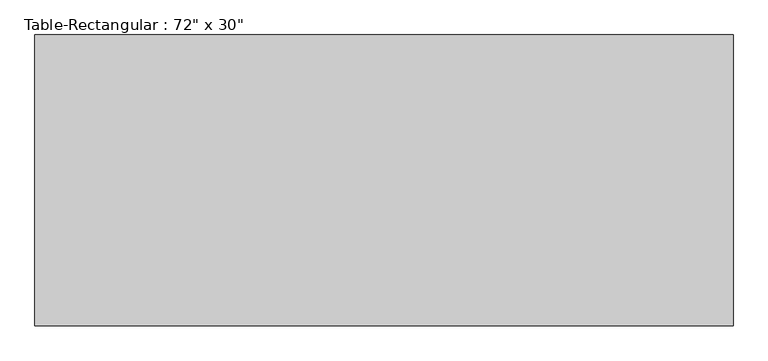
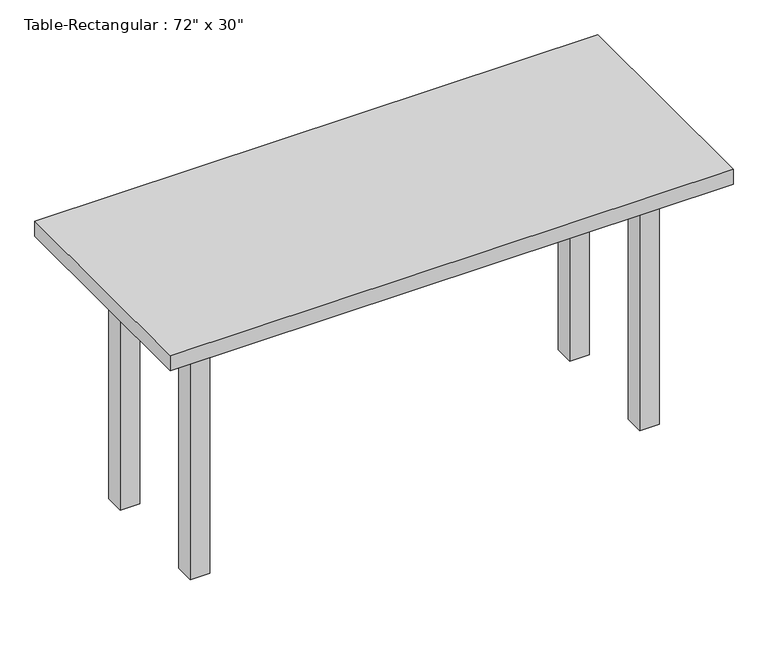
"""IFC4 building model written with IfcOpenShell, lengths in millimetres: furniture geometry."""

from ifc_helpers import new_model, si_unit, frame, origin, origin_with_axes, place, context, project, spatial, polyline, outline, extrude, source, transform, mapped, element, save


def furniture_046c8a23(model_context):
    return source(origin(), model_context, "Body", "SweptSolid", [
        extrude(outline(polyline([(698.5, 190.5), (698.5, 165.1), (-698.5, 165.1), (-698.5, 190.5), (698.5, 190.5)])), frame((0.0, 0.0, 762.0), z_axis=(0.0, 0.0, 1.0), x_axis=(1.0, 0.0, 0.0)), (0.0, 0.0, 1.0), 101.6),
        extrude(outline(polyline([(698.5, -190.5), (-698.5, -190.5), (-698.5, -165.1), (698.5, -165.1), (698.5, -190.5)])), frame((0.0, 0.0, 762.0), z_axis=(0.0, 0.0, 1.0), x_axis=(1.0, 0.0, 0.0)), (0.0, 0.0, 1.0), 101.6),
        extrude(outline(polyline([(-711.2, -165.1), (-736.6, -165.1), (-736.6, 165.1), (-711.2, 165.1), (-711.2, -165.1)])), frame((0.0, 0.0, 762.0), z_axis=(0.0, 0.0, 1.0), x_axis=(1.0, 0.0, 0.0)), (0.0, 0.0, 1.0), 101.6),
        extrude(outline(polyline([(711.2, -165.1), (711.2, 165.1), (736.6, 165.1), (736.6, -165.1), (711.2, -165.1)])), frame((0.0, 0.0, 762.0), z_axis=(0.0, 0.0, 1.0), x_axis=(1.0, 0.0, 0.0)), (0.0, 0.0, 1.0), 101.6),
        extrude(outline(polyline([(914.4, 381.0), (914.4, -381.0), (-914.4, -381.0), (-914.4, 381.0), (914.4, 381.0)])), frame((0.0, 0.0, 863.6), z_axis=(0.0, 0.0, 1.0), x_axis=(1.0, 0.0, 0.0)), (0.0, 0.0, 1.0), 50.8),
        extrude(outline(polyline([(-698.5, 228.6), (-698.5, 165.1), (-762.0, 165.1), (-762.0, 228.6), (-698.5, 228.6)])), origin_with_axes(), (0.0, 0.0, 1.0), 863.6),
        extrude(outline(polyline([(698.5, 228.6), (762.0, 228.6), (762.0, 165.1), (698.5, 165.1), (698.5, 228.6)])), origin_with_axes(), (0.0, 0.0, 1.0), 863.6),
        extrude(outline(polyline([(-698.5, -228.6), (-762.0, -228.6), (-762.0, -165.1), (-698.5, -165.1), (-698.5, -228.6)])), origin_with_axes(), (0.0, 0.0, 1.0), 863.6),
        extrude(outline(polyline([(698.5, -228.6), (698.5, -165.1), (762.0, -165.1), (762.0, -228.6), (698.5, -228.6)])), origin_with_axes(), (0.0, 0.0, 1.0), 863.6),
    ])


if __name__ == "__main__":
    model = new_model("IFC4")
    model_context = context("Model", 3, world=origin())
    ifc_project = project(units=[si_unit("LENGTHUNIT", "METRE", prefix="MILLI")], contexts=[model_context])
    site = spatial("IfcSite", under=ifc_project)
    building = spatial("IfcBuilding", under=site)
    placement = place(None, origin())
    furniture_shape = furniture_046c8a23(model_context)
    element("IfcFurniture", 1, ObjectType="Table-Rectangular : 72\" x 30\"", at=placement, inside=building, context=model_context, shape_type="MappedRepresentation", body=[
        mapped(furniture_shape, transform((0.0, 0.0, 0.0), x_axis=(1.0, 0.0, 0.0), y_axis=(0.0, 1.0, 0.0), z_axis=(0.0, 0.0, 1.0))),
    ])
    save(model, "model.ifc")

# Revit data of these elements
# Type "Table-Rectangular : 72\" x 30\""
#   Assembly Code = "E2020200"
#   Height = 3' - 0"
#   Length = 6' - 0"
#   Width = 2' - 6"
#   Base Material = Birch
#   Top Material = Birch
#   Default Elevation = 0
# Element 1 (IfcFurniture, "Table-Rectangular : 72\" x 30\"")
#   Materials on its faces: "Birch"
# Materials
#   "Birch": class "Wood", colour RGB 224 178 126, transparency 0, Description = "Betula Alleghaniensis", Cost = 0
